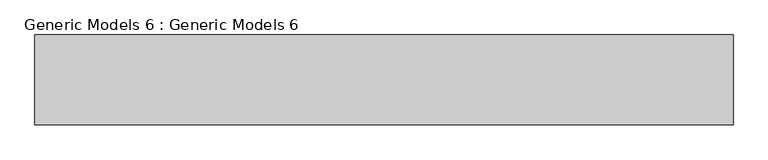
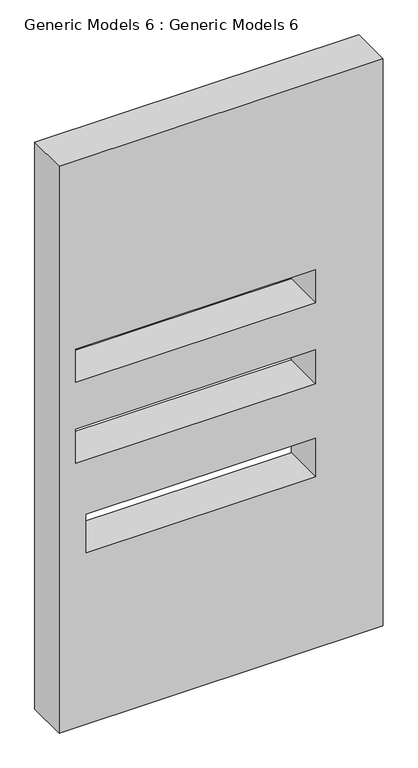
"""IFC4 building model written with IfcOpenShell, lengths in millimetres: proxy geometry, Generic Models 6 : Generic Models 6."""

from ifc_helpers import new_model, si_unit, frame, origin, place, context, project, spatial, polyline, outline, extrude, source, transform, mapped, element, save


def generic_models_6_generic_models_6_729a5b47(model_context):
    return source(origin(), model_context, "Body", "SweptSolid", [
        extrude(outline(polyline([(8144.858524, -11631.0356484), (8144.858524, -13997.6335986), (3769.3502296, -13997.6335986), (3769.3502296, -11631.0356484), (8144.858524, -11631.0356484)]), holes=[polyline([(6436.1698552, -12123.4171754), (6436.1698552, -13876.0171754), (6690.1698552, -13876.0171754), (6690.1698552, -12123.4171754), (6436.1698552, -12123.4171754)]), polyline([(5809.0263876, -12123.4171754), (5809.0263876, -13876.0171754), (6070.5063211, -13876.0171754), (6070.5063211, -12123.4171754), (5809.0263876, -12123.4171754)]), polyline([(5093.2773189, -12123.4171754), (5093.2773189, -13798.063152), (5388.9551907, -13798.063152), (5388.9551907, -12123.4171754), (5093.2773189, -12123.4171754)])]), frame((0.0, -4623.3088252, 0.0), z_axis=(0.0, 1.0, 0.0), x_axis=(0.0, 0.0, 1.0)), (0.0, 0.0, 1.0), 304.8),
    ])


if __name__ == "__main__":
    model = new_model("IFC4")
    model_context = context("Model", 3, world=origin())
    ifc_project = project(units=[si_unit("LENGTHUNIT", "METRE", prefix="MILLI")], contexts=[model_context])
    site = spatial("IfcSite", under=ifc_project)
    building = spatial("IfcBuilding", under=site)
    placement = place(None, origin())
    generic_models_6_generic_models_6_shape = generic_models_6_generic_models_6_729a5b47(model_context)
    element("IfcBuildingElementProxy", 1, Name="Generic Models 6 : Generic Models 6", ObjectType="Generic Models 6 : Generic Models 6", at=placement, inside=building, context=model_context, shape_type="MappedRepresentation", body=[
        mapped(generic_models_6_generic_models_6_shape, transform((0.0, 0.0, 0.0), x_axis=(1.0, 0.0, 0.0), y_axis=(0.0, 1.0, 0.0), z_axis=(0.0, 0.0, 1.0))),
    ])
    save(model, "model.ifc")
